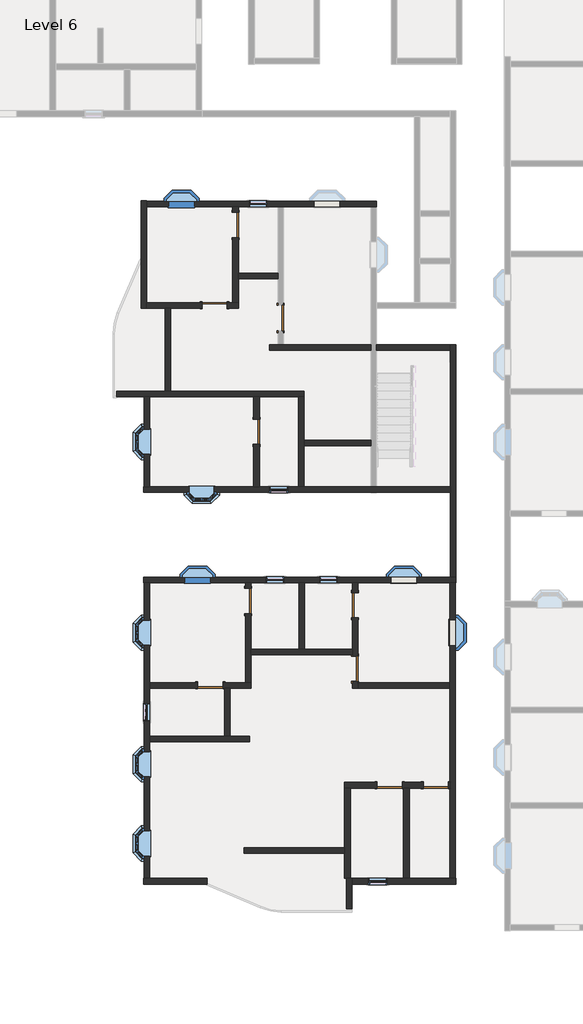
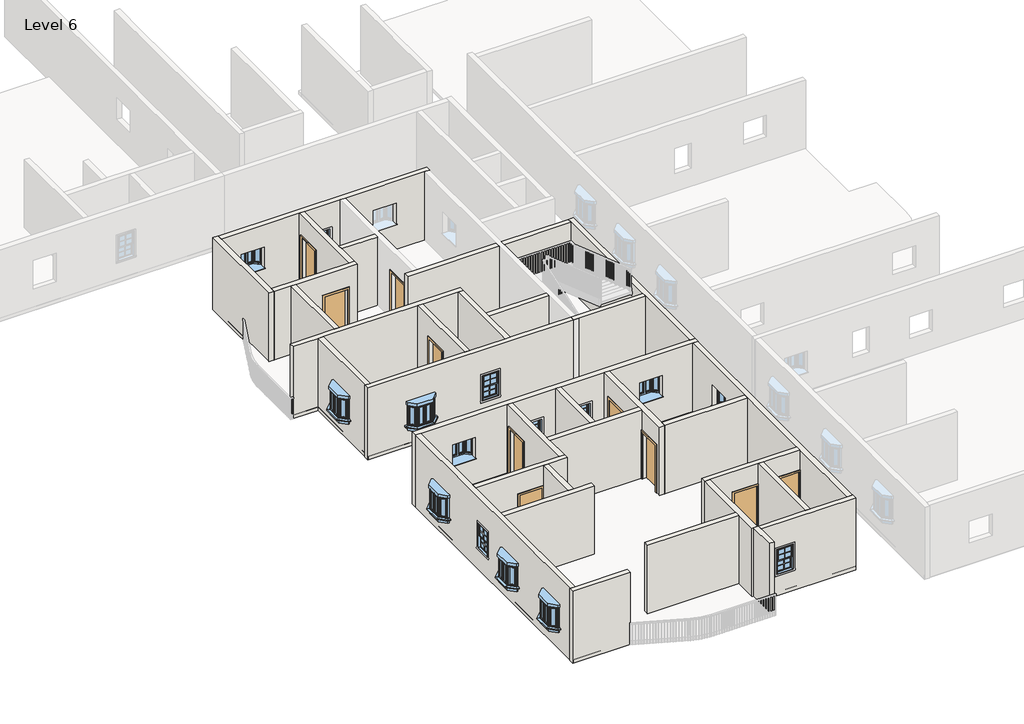
# One storey, part 1 of 14: 33 walls, 15 windows, 10 doors.
# Revit data of these elements (continued)
# Element 54 (IfcWindow, "Window-Double-Hung : 26\" x 42\"") (continued)
#   Window Inset = 0' - 0"
#   Interior Wall Closure = 0' - 1 1/2"
#   Frame Extension = 0' - 1 1/4"
#   Exterior Wall Closure = 0' - 0 1/2"
#   Interior Trim Visibility = yes
#   Indicator Visibility = yes
#   Exterior Trim Visibility = yes
#   Phase Created = New Construction
#   Materials on its faces: "Wood - Stained", "Glass", "Clad - White"
# Element 55 (IfcWindow, "Window-Double-Hung : 26\" x 42\"")
#   Mark = "352"
#   Window Inset = 0' - 0"
#   Interior Wall Closure = 0' - 1 1/2"
#   Frame Extension = 0' - 1 1/4"
#   Exterior Wall Closure = 0' - 0 1/2"
#   Interior Trim Visibility = yes
#   Indicator Visibility = yes
#   Exterior Trim Visibility = yes
#   Phase Created = New Construction
#   Materials on its faces: "Wood - Stained", "Glass", "Clad - White"
# Element 56 (IfcWindow, "Window-Double-Hung : 26\" x 42\"")
#   Mark = "353"
#   Window Inset = 0' - 0"
#   Interior Wall Closure = 0' - 1 1/2"
#   Frame Extension = 0' - 1 1/4"
#   Exterior Wall Closure = 0' - 0 1/2"
#   Interior Trim Visibility = yes
#   Indicator Visibility = yes
#   Exterior Trim Visibility = yes
#   Phase Created = New Construction
#   Materials on its faces: "Wood - Stained", "Glass", "Clad - White"
# Element 57 (IfcWindow, "Window-Double-Hung : 26\" x 42\"")
#   Mark = "354"
#   Window Inset = 0' - 0"
#   Interior Wall Closure = 0' - 1 1/2"
#   Frame Extension = 0' - 1 1/4"
#   Exterior Wall Closure = 0' - 0 1/2"
#   Interior Trim Visibility = yes
#   Indicator Visibility = yes
#   Exterior Trim Visibility = yes
#   Phase Created = New Construction
#   Materials on its faces: "Wood - Stained", "Glass", "Clad - White"
# Element 58 (IfcWindow, "Window-Double-Hung : 26\" x 42\"")
#   Mark = "355"
#   Window Inset = 0' - 0"
#   Interior Wall Closure = 0' - 1 1/2"
#   Frame Extension = 0' - 1 1/4"
#   Exterior Wall Closure = 0' - 0 1/2"
#   Interior Trim Visibility = yes
#   Indicator Visibility = yes
#   Exterior Trim Visibility = yes
#   Phase Created = New Construction
#   Materials on its faces: "Wood - Stained", "Glass", "Clad - White"
# Materials
#   "Door - Panel": class "Wood", colour RGB 210 159 95, transparency 0, Cost = 0
#   "Door - Frame": colour RGB 118 70 51, transparency 0, Cost = 0
#   "Window Frame": colour RGB 249 249 249, transparency 0
#   "Glass": class "Glass", colour RGB 0 128 192, transparency 0.75, Description = "Soda Lime Glass", Cost = 0
#   "Wood - Stained": class "Wood", colour RGB 224 178 126, transparency 0, Cost = 0
#   "Clad - White": class "Wood", colour RGB 242 242 238, transparency 0, Cost = 0
#   "Default Wall": colour RGB 128 128 128, transparency 0, Cost = 0
#   "Earth": class "Generic", colour RGB 97 75 62, transparency 0, Description = "Soil", Cost = 0
#   "Parking Stripe": class "Paint", colour RGB 250 250 91, transparency 0, Cost = 0
#   "Carpet (1)": class "Carpet", colour RGB 124 80 67, transparency 0, Description = "Interior finish", Cost = 0
#   "Softwood, Lumber": class "Wood", colour RGB 223 192 134, transparency 0, Description = "Pinus Echinata", Cost = 0
